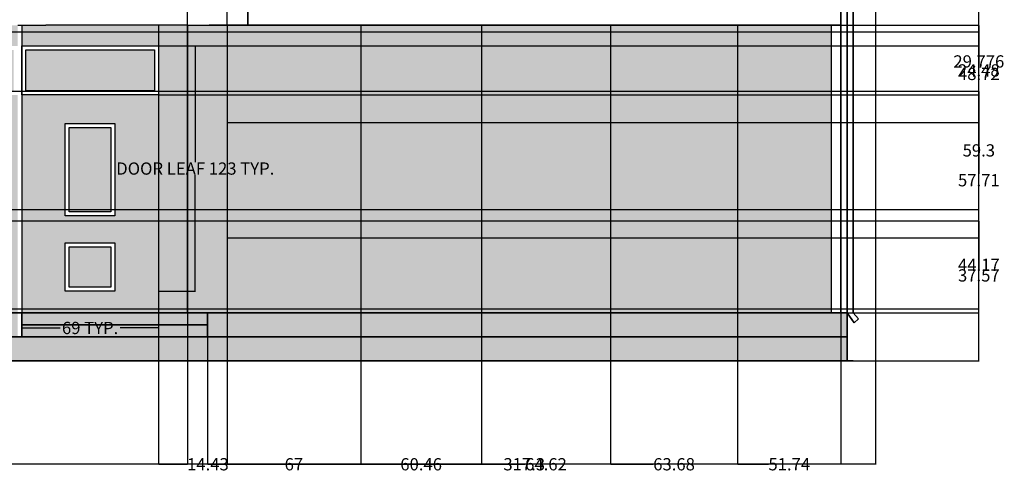
# Model space of a CAD drawing. Units: inches. Extents: x -655 to 499, y 20 to 616.
# Tile 6 of 7: x 5 to 499, y 20 to 246. Entities that reach past the tile are written whole.
import ezdxf

# ---------------------------------------------------------------- set-up
doc = ezdxf.new("R2010")
doc.units = ezdxf.units.IN
doc.header["$MEASUREMENT"] = 0
for name, color, linetype, lineweight in [('A-ANNO-DIMS', 2, 'Continuous', 18), ('A-DOOR', 4, 'Continuous', 25), ('A-ELEV', 7, 'Continuous', 35), ('A-ELEV-PATT', 9, 'Continuous', 13), ('A-GLAZ', 3, 'Continuous', 25), ('C-TOPO', 18, 'Continuous', 18)]:
    doc.layers.add(name, color=color, linetype=linetype, lineweight=lineweight)
doc.styles.get("Standard").update_dxf_attribs({"font": 'arial.ttf'})
doc.dimstyles.get("Standard").update_dxf_attribs({"dimtxt": 6.125, "dimasz": 0.18, "dimexe": 0.18, "dimexo": 0.0625, "dimgap": 0.09, "dimtad": 0, "dimtih": 1, "dimtoh": 1, "dimdec": 4, "dimzin": 0, "dimdsep": 46, "dimlunit": 4, "dimtxsty": 'Standard', "dimcen": 0.09, "dimadec": 0, "dimazin": 0, "dimtfac": 1, "dimtdec": 4, "dimtofl": 0, "dimtmove": 0, "dimatfit": 3, "dimfxl": 1, "dimtolj": 1, "dimtzin": 0, "dimarcsym": 0})

# ---------------------------------------------------------------- blocks, each defined once
blk = doc.blocks.new('DOOR-LEAF-PANEL')
for points in [[(0, 122.75), (68.54, 122.75), (68.54, 98.27), (0, 98.27)], [(2, 120.75), (66.54, 120.75), (66.54, 100.27), (2, 100.27)], [(21.82, 83.95), (46.58, 83.95), (46.58, 37.78), (21.82, 37.78)], [(23.82, 81.95), (44.58, 81.95), (44.58, 39.78), (23.82, 39.78)], [(21.82, 24.14), (46.58, 24.14), (46.58, 0), (21.82, 0)], [(23.82, 22.14), (44.58, 22.14), (44.58, 2), (23.82, 2)]]:
    blk.add_lwpolyline(points, close=True)
blk = doc.blocks.new('*D8')
at = {"layer": 'A-ANNO-DIMS', "color": 0, "lineweight": -2, "transparency": 16777216}
for p, q in [((75.03, 233.27), (93.56, 233.27)), ((93.38, 233.09), (93.38, 175.16)), ((93.38, 110.71), (93.38, 168.64)), ((75.03, 110.53), (93.56, 110.53))]:
    blk.add_line(p, q, dxfattribs=at)
at = {"layer": 'A-ANNO-DIMS', "color": 0, "transparency": 16777216}
for points in [[(93.35, 233.09), (93.41, 233.09), (93.38, 233.27)], [(93.35, 110.71), (93.41, 110.71), (93.38, 110.53)]]:
    blk.add_solid(points, dxfattribs=at)
at = {"layer": 'Defpoints', "color": 0, "transparency": 16777216}
for p in [(74.97, 233.27), (93.38, 233.27), (74.97, 110.53)]:
    blk.add_point(p, dxfattribs=at)
at = {"layer": 'A-ANNO-DIMS', "color": 0, "transparency": 16777216, "insert": (93.38, 171.9), "char_height": 6.125, "attachment_point": 5}
blk.add_mtext('\\A1;DOOR LEAF 123 TYP.', dxfattribs=at)
blk = doc.blocks.new('*D9')
at = {"layer": 'A-ANNO-DIMS', "color": 0, "lineweight": -2, "transparency": 16777216}
for p, q in [((6.43, 110.46), (6.43, 91.93)), ((74.97, 110.46), (74.97, 91.93)), ((6.61, 92.11), (25.68, 92.11)), ((74.79, 92.11), (55.71, 92.11))]:
    blk.add_line(p, q, dxfattribs=at)
at = {"layer": 'A-ANNO-DIMS', "color": 0, "transparency": 16777216}
for points in [[(6.61, 92.14), (6.61, 92.08), (6.43, 92.11)], [(74.79, 92.14), (74.79, 92.08), (74.97, 92.11)]]:
    blk.add_solid(points, dxfattribs=at)
at = {"layer": 'Defpoints', "color": 0, "transparency": 16777216}
for p in [(6.43, 110.53), (74.97, 110.53), (74.97, 92.11)]:
    blk.add_point(p, dxfattribs=at)
at = {"layer": 'A-ANNO-DIMS', "color": 0, "transparency": 16777216, "insert": (40.7, 92.11), "char_height": 6.125, "attachment_point": 5}
blk.add_mtext('\\A1;69 TYP.', dxfattribs=at)
blk = doc.blocks.new('*D10')
at = {"layer": 'A-ANNO-DIMS', "color": 0, "lineweight": -2, "transparency": 16777216}
for p, q in [((434.11, 393.11), (434.11, 23.7)), ((-590.16, 75.57), (-590.16, 23.7)), ((-589.98, 23.88), (-90.54, 23.88)), ((433.93, 23.88), (-65.51, 23.88))]:
    blk.add_line(p, q, dxfattribs=at)
at = {"layer": 'A-ANNO-DIMS', "color": 0, "transparency": 16777216}
for points in [[(-589.98, 23.91), (-589.98, 23.85), (-590.16, 23.88)], [(433.93, 23.91), (433.93, 23.85), (434.11, 23.88)]]:
    blk.add_solid(points, dxfattribs=at)
at = {"layer": 'Defpoints', "color": 0, "transparency": 16777216}
for p in [(434.11, 393.17), (-590.16, 75.63), (434.11, 23.88)]:
    blk.add_point(p, dxfattribs=at)
at = {"layer": 'A-ANNO-DIMS', "color": 0, "transparency": 16777216, "insert": (-78.02, 23.88), "char_height": 6.125, "attachment_point": 5}
blk.add_mtext('\\A1;1024.3', dxfattribs=at)
blk = doc.blocks.new('*D15')
at = {"layer": 'A-ANNO-DIMS', "color": 0, "lineweight": -2, "transparency": 16777216}
for p, q in [((-126.81, 99.57), (-126.81, 23.7)), ((99.5, 93.57), (99.5, 23.7)), ((-126.63, 23.88), (-24.13, 23.88)), ((99.32, 23.88), (-3.18, 23.88))]:
    blk.add_line(p, q, dxfattribs=at)
at = {"layer": 'A-ANNO-DIMS', "color": 0, "transparency": 16777216}
for points in [[(-126.63, 23.91), (-126.63, 23.85), (-126.81, 23.88)], [(99.32, 23.91), (99.32, 23.85), (99.5, 23.88)]]:
    blk.add_solid(points, dxfattribs=at)
at = {"layer": 'Defpoints', "color": 0, "transparency": 16777216}
for p in [(-126.81, 99.63), (99.5, 93.63), (99.5, 23.88)]:
    blk.add_point(p, dxfattribs=at)
at = {"layer": 'A-ANNO-DIMS', "color": 0, "transparency": 16777216, "insert": (-13.65, 23.88), "char_height": 6.125, "attachment_point": 5}
blk.add_mtext('\\A1;226.3', dxfattribs=at)
blk = doc.blocks.new('*D16')
at = {"layer": 'A-ANNO-DIMS', "color": 0, "lineweight": -2, "transparency": 16777216}
for p, q in [((416.78, 99.57), (416.78, 23.7)), ((99.5, 93.57), (99.5, 23.7)), ((99.68, 23.88), (247.71, 23.88)), ((416.6, 23.88), (268.56, 23.88))]:
    blk.add_line(p, q, dxfattribs=at)
at = {"layer": 'A-ANNO-DIMS', "color": 0, "transparency": 16777216}
for points in [[(99.68, 23.91), (99.68, 23.85), (99.5, 23.88)], [(416.6, 23.91), (416.6, 23.85), (416.78, 23.88)]]:
    blk.add_solid(points, dxfattribs=at)
at = {"layer": 'Defpoints', "color": 0, "transparency": 16777216}
for p in [(416.78, 99.63), (99.5, 93.63), (416.78, 23.88)]:
    blk.add_point(p, dxfattribs=at)
at = {"layer": 'A-ANNO-DIMS', "color": 0, "transparency": 16777216, "insert": (258.14, 23.88), "char_height": 6.125, "attachment_point": 5}
blk.add_mtext('\\A1;317.3', dxfattribs=at)
blk = doc.blocks.new('*D21')
at = {"layer": 'A-ANNO-DIMS', "color": 0, "lineweight": -2, "transparency": 16777216}
for p, q in [((179.11, 559.78), (486.04, 559.78)), ((485.86, 559.6), (485.86, 320.92)), ((485.86, 75.81), (485.86, 314.49)), ((-590.1, 75.63), (486.04, 75.63))]:
    blk.add_line(p, q, dxfattribs=at)
at = {"layer": 'A-ANNO-DIMS', "color": 0, "transparency": 16777216}
for points in [[(485.83, 559.6), (485.89, 559.6), (485.86, 559.78)], [(485.83, 75.81), (485.89, 75.81), (485.86, 75.63)]]:
    blk.add_solid(points, dxfattribs=at)
at = {"layer": 'Defpoints', "color": 0, "transparency": 16777216}
for p in [(179.05, 559.78), (485.86, 559.78), (-590.16, 75.63)]:
    blk.add_point(p, dxfattribs=at)
at = {"layer": 'A-ANNO-DIMS', "color": 0, "transparency": 16777216, "insert": (485.86, 317.7), "char_height": 6.125, "attachment_point": 5}
blk.add_mtext('\\A1;484.15', dxfattribs=at)
blk = doc.blocks.new('*D48')
at = {"layer": 'A-ANNO-DIMS', "color": 0, "lineweight": -2, "transparency": 16777216}
for p, q in [((-228.95, 145.8), (486.04, 145.8)), ((485.86, 145.62), (485.86, 126.88)), ((485.86, 101.81), (485.86, 120.55)), ((-228.95, 101.63), (486.04, 101.63))]:
    blk.add_line(p, q, dxfattribs=at)
at = {"layer": 'A-ANNO-DIMS', "color": 0, "transparency": 16777216}
for points in [[(485.83, 145.62), (485.89, 145.62), (485.86, 145.8)], [(485.83, 101.81), (485.89, 101.81), (485.86, 101.63)]]:
    blk.add_solid(points, dxfattribs=at)
at = {"layer": 'Defpoints', "color": 0, "transparency": 16777216}
for p in [(-229.01, 145.8), (485.86, 145.8), (-229.01, 101.63)]:
    blk.add_point(p, dxfattribs=at)
at = {"layer": 'A-ANNO-DIMS', "color": 0, "transparency": 16777216, "insert": (485.86, 123.72), "char_height": 6.125, "attachment_point": 5}
blk.add_mtext('\\A1;44.17', dxfattribs=at)
blk = doc.blocks.new('*D49')
at = {"layer": 'A-ANNO-DIMS', "color": 0, "lineweight": -2, "transparency": 16777216}
for p, q in [((-229.3, 210.64), (486.04, 210.64)), ((485.86, 210.46), (485.86, 184.21)), ((485.86, 151.52), (485.86, 177.77)), ((-229.3, 151.34), (486.04, 151.34))]:
    blk.add_line(p, q, dxfattribs=at)
at = {"layer": 'A-ANNO-DIMS', "color": 0, "transparency": 16777216}
for points in [[(485.83, 210.46), (485.89, 210.46), (485.86, 210.64)], [(485.83, 151.52), (485.89, 151.52), (485.86, 151.34)]]:
    blk.add_solid(points, dxfattribs=at)
at = {"layer": 'Defpoints', "color": 0, "transparency": 16777216}
for p in [(-229.36, 210.64), (485.86, 210.64), (-229.36, 151.34)]:
    blk.add_point(p, dxfattribs=at)
at = {"layer": 'A-ANNO-DIMS', "color": 0, "transparency": 16777216, "insert": (485.86, 180.99), "char_height": 6.125, "attachment_point": 5}
blk.add_mtext('\\A1;59.3', dxfattribs=at)
blk = doc.blocks.new('*D51')
at = {"layer": 'A-ANNO-DIMS', "color": 0, "lineweight": -2, "transparency": 16777216}
for p, q in [((-228.95, 240.42), (486.04, 240.42)), ((485.86, 240.24), (485.86, 228.75)), ((485.86, 210.82), (485.86, 222.31)), ((-228.88, 210.64), (486.04, 210.64))]:
    blk.add_line(p, q, dxfattribs=at)
at = {"layer": 'A-ANNO-DIMS', "color": 0, "transparency": 16777216}
for points in [[(485.83, 240.24), (485.89, 240.24), (485.86, 240.42)], [(485.83, 210.82), (485.89, 210.82), (485.86, 210.64)]]:
    blk.add_solid(points, dxfattribs=at)
at = {"layer": 'Defpoints', "color": 0, "transparency": 16777216}
for p in [(-229.01, 240.42), (485.86, 240.42), (-228.94, 210.64)]:
    blk.add_point(p, dxfattribs=at)
at = {"layer": 'A-ANNO-DIMS', "color": 0, "transparency": 16777216, "insert": (485.86, 225.53), "char_height": 6.125, "attachment_point": 5}
blk.add_mtext('\\A1;29.776', dxfattribs=at)
blk = doc.blocks.new('*D61')
at = {"layer": 'A-ANNO-DIMS', "color": 0, "lineweight": -2, "transparency": 16777216}
for p, q in [((-64.12, 233.34), (-64.12, 611.71)), ((89.4, 243.69), (89.4, 611.71)), ((-63.94, 611.53), (0.16, 611.53)), ((89.22, 611.53), (25.13, 611.53))]:
    blk.add_line(p, q, dxfattribs=at)
at = {"layer": 'A-ANNO-DIMS', "color": 0, "transparency": 16777216}
for points in [[(-63.94, 611.56), (-63.94, 611.5), (-64.12, 611.53)], [(89.22, 611.56), (89.22, 611.5), (89.4, 611.53)]]:
    blk.add_solid(points, dxfattribs=at)
at = {"layer": 'Defpoints', "color": 0, "transparency": 16777216}
for p in [(89.4, 611.53), (89.4, 243.63), (-64.12, 233.27)]:
    blk.add_point(p, dxfattribs=at)
at = {"layer": 'A-ANNO-DIMS', "color": 0, "transparency": 16777216, "insert": (12.64, 611.53), "char_height": 6.125, "attachment_point": 5}
blk.add_mtext('\\A1;153.52', dxfattribs=at)
blk = doc.blocks.new('*D62')
at = {"layer": 'A-ANNO-DIMS', "color": 0, "lineweight": -2, "transparency": 16777216}
for p, q in [((89.4, 243.69), (89.4, 611.71)), ((109.28, 243.69), (109.28, 611.71)), ((89.58, 611.53), (109.1, 611.53)), ((109.28, 611.53), (109.46, 611.53))]:
    blk.add_line(p, q, dxfattribs=at)
at = {"layer": 'A-ANNO-DIMS', "color": 0, "transparency": 16777216}
for points in [[(89.58, 611.56), (89.58, 611.5), (89.4, 611.53)], [(109.1, 611.56), (109.1, 611.5), (109.28, 611.53)]]:
    blk.add_solid(points, dxfattribs=at)
at = {"layer": 'Defpoints', "color": 0, "transparency": 16777216}
for p in [(109.28, 611.53), (89.4, 243.63), (109.28, 243.63)]:
    blk.add_point(p, dxfattribs=at)
at = {"layer": 'A-ANNO-DIMS', "color": 0, "transparency": 16777216, "insert": (121.99, 611.53), "char_height": 6.125, "attachment_point": 5}
blk.add_mtext('\\A1;19.875', dxfattribs=at)
blk = doc.blocks.new('*D63')
at = {"layer": 'A-ANNO-DIMS', "color": 0, "lineweight": -2, "transparency": 16777216}
for p, q in [((74.97, 99.57), (74.97, 23.7)), ((89.4, 99.57), (89.4, 23.7)), ((75.15, 23.88), (89.22, 23.88)), ((89.4, 23.88), (89.58, 23.88))]:
    blk.add_line(p, q, dxfattribs=at)
at = {"layer": 'A-ANNO-DIMS', "color": 0, "transparency": 16777216}
for points in [[(75.15, 23.91), (75.15, 23.85), (74.97, 23.88)], [(89.22, 23.91), (89.22, 23.85), (89.4, 23.88)]]:
    blk.add_solid(points, dxfattribs=at)
at = {"layer": 'Defpoints', "color": 0, "transparency": 16777216}
for p in [(74.97, 99.63), (89.4, 99.63), (89.4, 23.88)]:
    blk.add_point(p, dxfattribs=at)
at = {"layer": 'A-ANNO-DIMS', "color": 0, "transparency": 16777216, "insert": (99.72, 23.88), "char_height": 6.125, "attachment_point": 5}
blk.add_mtext('\\A1;14.43', dxfattribs=at)
blk = doc.blocks.new('*D64')
at = {"layer": 'A-ANNO-DIMS', "color": 0, "lineweight": -2, "transparency": 16777216}
for p, q in [((75.03, 233.27), (486.04, 233.27)), ((485.86, 233.09), (485.86, 224.25)), ((485.86, 208.97), (485.86, 217.82)), ((75.03, 208.79), (486.04, 208.79))]:
    blk.add_line(p, q, dxfattribs=at)
at = {"layer": 'A-ANNO-DIMS', "color": 0, "transparency": 16777216}
for points in [[(485.83, 233.09), (485.89, 233.09), (485.86, 233.27)], [(485.83, 208.97), (485.89, 208.97), (485.86, 208.79)]]:
    blk.add_solid(points, dxfattribs=at)
at = {"layer": 'Defpoints', "color": 0, "transparency": 16777216}
for p in [(74.97, 233.27), (485.86, 233.27), (74.97, 208.79)]:
    blk.add_point(p, dxfattribs=at)
at = {"layer": 'A-ANNO-DIMS', "color": 0, "transparency": 16777216, "insert": (485.86, 221.03), "char_height": 6.125, "attachment_point": 5}
blk.add_mtext('\\A1;24.48', dxfattribs=at)
blk = doc.blocks.new('*D72')
at = {"layer": 'A-ANNO-DIMS', "color": 0, "lineweight": -2, "transparency": 16777216}
for p, q in [((109.28, 243.57), (109.28, 23.7)), ((176.28, 243.57), (176.28, 23.7)), ((109.46, 23.88), (138.28, 23.88)), ((176.1, 23.88), (147.27, 23.88))]:
    blk.add_line(p, q, dxfattribs=at)
at = {"layer": 'A-ANNO-DIMS', "color": 0, "transparency": 16777216}
for points in [[(109.46, 23.91), (109.46, 23.85), (109.28, 23.88)], [(176.1, 23.91), (176.1, 23.85), (176.28, 23.88)]]:
    blk.add_solid(points, dxfattribs=at)
at = {"layer": 'Defpoints', "color": 0, "transparency": 16777216}
for p in [(109.28, 243.63), (176.28, 243.63), (176.28, 23.88)]:
    blk.add_point(p, dxfattribs=at)
at = {"layer": 'A-ANNO-DIMS', "color": 0, "transparency": 16777216, "insert": (142.78, 23.88), "char_height": 6.125, "attachment_point": 5}
blk.add_mtext('\\A1;67', dxfattribs=at)
blk = doc.blocks.new('*D73')
at = {"layer": 'A-ANNO-DIMS', "color": 0, "lineweight": -2, "transparency": 16777216}
for p, q in [((176.28, 243.57), (176.28, 23.7)), ((236.74, 243.57), (236.74, 23.7)), ((176.46, 23.88), (196.07, 23.88)), ((236.56, 23.88), (216.95, 23.88))]:
    blk.add_line(p, q, dxfattribs=at)
at = {"layer": 'A-ANNO-DIMS', "color": 0, "transparency": 16777216}
for points in [[(176.46, 23.91), (176.46, 23.85), (176.28, 23.88)], [(236.56, 23.91), (236.56, 23.85), (236.74, 23.88)]]:
    blk.add_solid(points, dxfattribs=at)
at = {"layer": 'Defpoints', "color": 0, "transparency": 16777216}
for p in [(176.28, 243.63), (236.74, 243.63), (236.74, 23.88)]:
    blk.add_point(p, dxfattribs=at)
at = {"layer": 'A-ANNO-DIMS', "color": 0, "transparency": 16777216, "insert": (206.51, 23.88), "char_height": 6.125, "attachment_point": 5}
blk.add_mtext('\\A1;60.46', dxfattribs=at)
blk = doc.blocks.new('*D74')
at = {"layer": 'A-ANNO-DIMS', "color": 0, "lineweight": -2, "transparency": 16777216}
for p, q in [((236.74, 243.57), (236.74, 23.7)), ((301.36, 243.57), (301.36, 23.7)), ((236.92, 23.88), (258.64, 23.88)), ((301.18, 23.88), (279.46, 23.88))]:
    blk.add_line(p, q, dxfattribs=at)
at = {"layer": 'A-ANNO-DIMS', "color": 0, "transparency": 16777216}
for points in [[(236.92, 23.91), (236.92, 23.85), (236.74, 23.88)], [(301.18, 23.91), (301.18, 23.85), (301.36, 23.88)]]:
    blk.add_solid(points, dxfattribs=at)
at = {"layer": 'Defpoints', "color": 0, "transparency": 16777216}
for p in [(236.74, 243.63), (301.36, 243.63), (301.36, 23.88)]:
    blk.add_point(p, dxfattribs=at)
at = {"layer": 'A-ANNO-DIMS', "color": 0, "transparency": 16777216, "insert": (269.05, 23.88), "char_height": 6.125, "attachment_point": 5}
blk.add_mtext('\\A1;64.62', dxfattribs=at)
blk = doc.blocks.new('*D75')
at = {"layer": 'A-ANNO-DIMS', "color": 0, "lineweight": -2, "transparency": 16777216}
for p, q in [((301.36, 243.57), (301.36, 23.7)), ((365.04, 243.57), (365.04, 23.7)), ((301.54, 23.88), (322.75, 23.88)), ((364.86, 23.88), (343.65, 23.88))]:
    blk.add_line(p, q, dxfattribs=at)
at = {"layer": 'A-ANNO-DIMS', "color": 0, "transparency": 16777216}
for points in [[(301.54, 23.91), (301.54, 23.85), (301.36, 23.88)], [(364.86, 23.91), (364.86, 23.85), (365.04, 23.88)]]:
    blk.add_solid(points, dxfattribs=at)
at = {"layer": 'Defpoints', "color": 0, "transparency": 16777216}
for p in [(301.36, 243.63), (365.04, 243.63), (365.04, 23.88)]:
    blk.add_point(p, dxfattribs=at)
at = {"layer": 'A-ANNO-DIMS', "color": 0, "transparency": 16777216, "insert": (333.2, 23.88), "char_height": 6.125, "attachment_point": 5}
blk.add_mtext('\\A1;63.68', dxfattribs=at)
blk = doc.blocks.new('*D76')
at = {"layer": 'A-ANNO-DIMS', "color": 0, "lineweight": -2, "transparency": 16777216}
for p, q in [((365.04, 243.57), (365.04, 23.7)), ((416.78, 243.57), (416.78, 23.7)), ((365.22, 23.88), (380.5, 23.88)), ((416.6, 23.88), (401.32, 23.88))]:
    blk.add_line(p, q, dxfattribs=at)
at = {"layer": 'A-ANNO-DIMS', "color": 0, "transparency": 16777216}
for points in [[(365.22, 23.91), (365.22, 23.85), (365.04, 23.88)], [(416.6, 23.91), (416.6, 23.85), (416.78, 23.88)]]:
    blk.add_solid(points, dxfattribs=at)
at = {"layer": 'Defpoints', "color": 0, "transparency": 16777216}
for p in [(365.04, 243.63), (416.78, 243.63), (416.78, 23.88)]:
    blk.add_point(p, dxfattribs=at)
at = {"layer": 'A-ANNO-DIMS', "color": 0, "transparency": 16777216, "insert": (390.91, 23.88), "char_height": 6.125, "attachment_point": 5}
blk.add_mtext('\\A1;51.74', dxfattribs=at)
blk = doc.blocks.new('*D77')
at = {"layer": 'A-ANNO-DIMS', "color": 0, "lineweight": -2, "transparency": 16777216}
for p, q in [((412.05, 137.2), (486.04, 137.2)), ((485.86, 137.02), (485.86, 121.63)), ((485.86, 99.81), (485.86, 115.2)), ((416.84, 99.63), (486.04, 99.63))]:
    blk.add_line(p, q, dxfattribs=at)
at = {"layer": 'A-ANNO-DIMS', "color": 0, "transparency": 16777216}
for points in [[(485.83, 137.02), (485.89, 137.02), (485.86, 137.2)], [(485.83, 99.81), (485.89, 99.81), (485.86, 99.63)]]:
    blk.add_solid(points, dxfattribs=at)
at = {"layer": 'Defpoints', "color": 0, "transparency": 16777216}
for p in [(411.99, 137.2), (485.86, 137.2), (416.78, 99.63)]:
    blk.add_point(p, dxfattribs=at)
at = {"layer": 'A-ANNO-DIMS', "color": 0, "transparency": 16777216, "insert": (485.86, 118.41), "char_height": 6.125, "attachment_point": 5}
blk.add_mtext('\\A1;37.57', dxfattribs=at)
blk = doc.blocks.new('*D78')
at = {"layer": 'A-ANNO-DIMS', "color": 0, "lineweight": -2, "transparency": 16777216}
for p, q in [((412.05, 194.91), (486.04, 194.91)), ((485.86, 194.73), (485.86, 169.27)), ((485.86, 137.38), (485.86, 162.84)), ((412.05, 137.2), (486.04, 137.2))]:
    blk.add_line(p, q, dxfattribs=at)
at = {"layer": 'A-ANNO-DIMS', "color": 0, "transparency": 16777216}
for points in [[(485.83, 194.73), (485.89, 194.73), (485.86, 194.91)], [(485.83, 137.38), (485.89, 137.38), (485.86, 137.2)]]:
    blk.add_solid(points, dxfattribs=at)
at = {"layer": 'Defpoints', "color": 0, "transparency": 16777216}
for p in [(411.99, 194.91), (485.86, 194.91), (411.99, 137.2)]:
    blk.add_point(p, dxfattribs=at)
at = {"layer": 'A-ANNO-DIMS', "color": 0, "transparency": 16777216, "insert": (485.86, 166.06), "char_height": 6.125, "attachment_point": 5}
blk.add_mtext('\\A1;57.71', dxfattribs=at)
blk = doc.blocks.new('*D79')
at = {"layer": 'A-ANNO-DIMS', "color": 0, "lineweight": -2, "transparency": 16777216}
for p, q in [((416.84, 243.63), (486.04, 243.63)), ((485.86, 243.45), (485.86, 222.49)), ((485.86, 195.09), (485.86, 216.05)), ((412.05, 194.91), (486.04, 194.91))]:
    blk.add_line(p, q, dxfattribs=at)
at = {"layer": 'A-ANNO-DIMS', "color": 0, "transparency": 16777216}
for points in [[(485.83, 243.45), (485.89, 243.45), (485.86, 243.63)], [(485.83, 195.09), (485.89, 195.09), (485.86, 194.91)]]:
    blk.add_solid(points, dxfattribs=at)
at = {"layer": 'Defpoints', "color": 0, "transparency": 16777216}
for p in [(416.78, 243.63), (485.86, 243.63), (411.99, 194.91)]:
    blk.add_point(p, dxfattribs=at)
at = {"layer": 'A-ANNO-DIMS', "color": 0, "transparency": 16777216, "insert": (485.86, 219.27), "char_height": 6.125, "attachment_point": 5}
blk.add_mtext('\\A1;48.72', dxfattribs=at)
blk = doc.blocks.new('*D80')
at = {"layer": 'A-ANNO-DIMS', "color": 0, "lineweight": -2, "transparency": 16777216}
for p, q in [((270.7, 282.96), (486.04, 282.96)), ((485.86, 282.78), (485.86, 266.51)), ((485.86, 243.81), (485.86, 260.07)), ((416.84, 243.63), (486.04, 243.63))]:
    blk.add_line(p, q, dxfattribs=at)
at = {"layer": 'A-ANNO-DIMS', "color": 0, "transparency": 16777216}
for points in [[(485.83, 282.78), (485.89, 282.78), (485.86, 282.96)], [(485.83, 243.81), (485.89, 243.81), (485.86, 243.63)]]:
    blk.add_solid(points, dxfattribs=at)
at = {"layer": 'Defpoints', "color": 0, "transparency": 16777216}
for p in [(270.64, 282.96), (485.86, 282.96), (416.78, 243.63)]:
    blk.add_point(p, dxfattribs=at)
at = {"layer": 'A-ANNO-DIMS', "color": 0, "transparency": 16777216, "insert": (485.86, 263.29), "char_height": 6.125, "attachment_point": 5}
blk.add_mtext('\\A1;39.33', dxfattribs=at)

msp = doc.modelspace()

# ---------------------------------------------------------------- hatches: boundary and pattern name
at = {"layer": 'A-ELEV-PATT'}
h = msp.add_hatch(color=256, dxfattribs=at)
h.dxf.hatch_style = 1
h.paths.add_polyline_path([(-140.0489, 272.2618), (-399.3758, 272.2618), (-399.3758, 249.8418), (-399.3758, 248.5179), (-366.9446, 248.7444), (-209.8047, 249.8418), (-183.5755, 249.8418), (-140.0489, 249.8418)])
h.paths.add_polyline_path([(-211.7589, 317.0515), (-216.5713, 317.0515), (-216.5713, 272.2618), (-211.7589, 272.2618)])
h.paths.add_polyline_path([(-145.96, 317.0515), (-150.7725, 317.0515), (-150.7725, 272.2618), (-145.96, 272.2618)])
h.paths.add_polyline_path([(-140.5198, 321.4867), (-402.0739, 321.4867), (-402.0739, 317.0515), (-390.1757, 317.0515), (-385.3633, 317.0515), (-150.7725, 317.0515), (-145.96, 317.0515), (-140.5198, 317.0515)])
h.paths.add_polyline_path([(-269.7123, 317.0515), (-274.5248, 317.0515), (-274.5248, 272.2618), (-269.7123, 272.2618)])
h.paths.add_polyline_path([(-329.7837, 317.0515), (-334.5961, 317.0515), (-334.5961, 280.9678), (-329.7837, 280.9678)])
h.paths.add_polyline_path([(-329.7837, 280.9678), (-334.5961, 280.9678), (-334.5961, 272.2618), (-329.7837, 272.2618)])
h.paths.add_polyline_path([(-385.3633, 317.0515), (-390.1757, 317.0515), (-390.1757, 272.2618), (-385.3633, 272.2618)])
h.paths.add_polyline_path([(-229.0087, 240.4184), (-354.3532, 240.4184), (-354.2854, 210.6425), (-315.9956, 210.6425), (-315.9956, 210.9348), (-277.6793, 210.7995), (-277.6793, 210.6425), (-273.1052, 210.6425), (-273.1052, 210.7995), (-229.3637, 210.6425), (-229.0087, 210.6425)])
h.paths.add_polyline_path([(-229.0087, 145.8007), (-354.3532, 145.8007), (-354.3532, 101.6296), (-229.0087, 101.6296)])
h.paths.add_polyline_path([(-229.0087, 210.6425), (-229.3637, 210.6425), (-229.3637, 151.3385), (-273.1052, 151.4955), (-273.1052, 210.6425), (-277.6793, 210.6425), (-277.6793, 151.4955), (-315.9956, 151.6308), (-315.9956, 210.6425), (-318.9742, 210.6425), (-318.9742, 151.3385), (-354.3532, 151.3385), (-354.3532, 145.8007), (-229.0087, 145.8007)])
h.paths.add_polyline_path([(-229.0087, 247.8418), (-354.3532, 247.8418), (-354.3532, 240.4184), (-229.0087, 240.4184)])
h.paths.add_polyline_path([(4.4271, 93.6296), (-100.4134, 93.6296), (-124.8077, 93.6296), (-126.8077, 93.6296), (-126.8077, 87.6296), (4.4271, 87.6296)])
h.paths.add_polyline_path([(4.4271, 99.6296), (-100.4134, 99.6296), (-100.4134, 93.6296), (4.4271, 93.6296)])
h.paths.add_polyline_path([(99.4982, 99.6296), (6.4271, 99.6296), (6.4271, 93.6296), (99.4982, 93.6296)])
h.paths.add_polyline_path([(99.4982, 93.6296), (6.4271, 93.6296), (6.4271, 87.6296), (99.4982, 87.6296)])
h.paths.add_polyline_path([(304.2843, 311.436), (230.0144, 311.076), (230.0144, 282.9577), (270.6361, 282.9577), (304.4665, 273.8535)])
h.paths.add_polyline_path([(304.1054, 348.3371), (304.1054, 356.2861), (230.0144, 356.2861), (230.0144, 348.3443), (230.0144, 311.076), (304.2843, 311.436)])
h.paths.add_polyline_path([(255.5586, 316.5111), (255.5586, 350.0185), (275.6848, 350.0185), (275.6848, 316.5111)], flags=16)
h.paths.add_polyline_path([(278.0676, 316.5111), (278.0676, 350.0185), (301.4074, 350.0185), (301.4074, 316.5111)], flags=16)
h.paths.add_polyline_path([(253.2029, 316.5111), (233.8107, 316.5111), (233.8107, 350.0185), (253.2029, 350.0185)], flags=16)
h.paths.add_polyline_path([(179.0482, 559.7795), (153.2347, 535.8185), (165.0976, 535.8185), (192.9989, 535.8185), (201.2897, 535.8185)])
h.paths.add_polyline_path([(347.8163, 516.7932), (322.0028, 492.8322), (333.8657, 492.8322), (361.7669, 492.8322), (370.0577, 492.8322)])
h = msp.add_hatch(color=256, dxfattribs=at)
h.dxf.hatch_style = 1
h.paths.add_polyline_path([(-329.7837, 350.1333), (-347.0336, 350.1333), (-347.0336, 321.4867), (-329.7837, 321.4867)])
h.paths.add_polyline_path([(-294.1413, 350.1333), (-311.3912, 350.1333), (-311.3912, 321.4867), (-294.1413, 321.4867)])
h.paths.add_polyline_path([(-294.1413, 317.0515), (-311.3912, 317.0515), (-311.3912, 280.9678), (-294.1413, 280.9678)])
h.paths.add_polyline_path([(-334.5961, 317.0515), (-347.0336, 317.0515), (-347.0336, 280.9678), (-334.5961, 280.9678)])
h.paths.add_polyline_path([(-244.6859, 336.719), (-258.4486, 336.719), (-258.4486, 347.0139), (-244.6859, 347.0139), (-244.6859, 350.1333), (-261.9358, 350.1333), (-261.9358, 321.4867), (-244.6859, 321.4867)])
h.paths.add_polyline_path([(-244.6859, 317.0515), (-261.9358, 317.0515), (-261.9358, 280.9678), (-244.6859, 280.9678)])
h.paths.add_polyline_path([(-244.6859, 347.0139), (-258.4486, 347.0139), (-258.4486, 336.719), (-244.6859, 336.719)], flags=17)
h.paths.add_polyline_path([(-318.9742, 210.6425), (-354.3532, 210.6425), (-354.3532, 151.3385), (-318.9742, 151.3385)])
h.paths.add_polyline_path([(-277.6793, 210.6425), (-315.9956, 210.6425), (-315.9956, 151.6308), (-277.6793, 151.4955)])
h.paths.add_polyline_path([(-229.3637, 210.6425), (-273.1052, 210.6425), (-273.1052, 151.4955), (-229.3637, 151.3385)])
h.paths.add_polyline_path([(-19.537, 192.4712), (-40.2951, 192.4712), (-40.2951, 150.3082), (-19.537, 150.3082)])
h.paths.add_polyline_path([(2.4271, 231.274), (-62.1158, 231.274), (-62.1158, 210.7923), (2.4271, 210.7923)])
h.paths.add_polyline_path([(72.97, 231.274), (8.4271, 231.274), (8.4271, 210.7923), (72.97, 210.7923)])
h.paths.add_polyline_path([(51.0059, 192.4712), (30.2478, 192.4712), (30.2478, 150.3082), (51.0059, 150.3082)])
h.paths.add_polyline_path([(51.0059, 132.6671), (30.2478, 132.6671), (30.2478, 112.5254), (51.0059, 112.5254)])
h.paths.add_polyline_path([(-19.537, 132.6671), (-40.2951, 132.6671), (-40.2951, 112.5254), (-19.537, 112.5254)])
h.paths.add_polyline_path([(275.6848, 350.0185), (255.5586, 350.0185), (255.5586, 316.5111), (275.6848, 316.5111)])
h.paths.add_polyline_path([(301.4074, 350.0185), (278.0676, 350.0185), (278.0676, 316.5111), (301.4074, 316.5111)])
h.paths.add_polyline_path([(253.2029, 350.0185), (233.8107, 350.0185), (233.8107, 316.5111), (253.2029, 316.5111)])
h = msp.add_hatch(color=256, dxfattribs=at)
h.dxf.hatch_style = 1
h.paths.add_polyline_path([(-150.7725, 317.0515), (-211.7589, 317.0515), (-211.7589, 272.2618), (-150.7725, 272.2618)])
h.paths.add_polyline_path([(-229.0087, 317.0515), (-244.6859, 317.0515), (-244.6859, 280.9678), (-261.9358, 280.9678), (-261.9358, 317.0515), (-269.7123, 317.0515), (-269.7123, 272.2618), (-229.0087, 272.2618)])
h.paths.add_polyline_path([(-216.5713, 317.0515), (-227.0087, 317.0515), (-227.0087, 272.2618), (-216.5713, 272.2618)])
h.paths.add_polyline_path([(-274.5248, 317.0515), (-294.1413, 317.0515), (-294.1413, 280.9678), (-311.3912, 280.9678), (-311.3912, 317.0515), (-329.7837, 317.0515), (-329.7837, 280.9678), (-329.7837, 272.2618), (-274.5248, 272.2618)])
h.paths.add_polyline_path([(-347.0336, 317.0515), (-355.429, 317.0515), (-355.429, 272.2618), (-334.5961, 272.2618), (-334.5961, 280.9678), (-347.0336, 280.9678)])
h.paths.add_polyline_path([(-357.429, 317.0515), (-385.3633, 317.0515), (-385.3633, 272.2618), (-357.429, 272.2618)])
h.paths.add_polyline_path([(176.2798, 243.6296), (109.2763, 243.6296), (109.2763, 194.9112), (176.2798, 194.9112)])
h.paths.add_polyline_path([(176.2798, 194.9112), (109.2763, 194.9112), (109.2763, 137.2003), (176.2798, 137.2003)])
h.paths.add_polyline_path([(236.7365, 243.6296), (176.2798, 243.6296), (176.2798, 194.9112), (236.7365, 194.9112)])
h.paths.add_polyline_path([(236.7365, 194.9112), (176.2798, 194.9112), (176.2798, 137.2003), (236.7365, 137.2003)])
h.paths.add_polyline_path([(236.7365, 137.2003), (176.2798, 137.2003), (176.2798, 99.6296), (236.7365, 99.6296)])
h.paths.add_polyline_path([(176.2798, 137.2003), (109.2763, 137.2003), (109.2763, 99.6296), (176.2798, 99.6296)])
h.paths.add_polyline_path([(301.3566, 137.2003), (236.7365, 137.2003), (236.7365, 99.6296), (301.3566, 99.6296)])
h.paths.add_polyline_path([(301.3566, 194.9112), (236.7365, 194.9112), (236.7365, 137.2003), (301.3566, 137.2003)])
h.paths.add_polyline_path([(301.3566, 243.6296), (236.7365, 243.6296), (236.7365, 194.9112), (301.3566, 194.9112)])
h.paths.add_polyline_path([(365.0401, 243.6296), (301.3566, 243.6296), (301.3566, 194.9112), (365.0401, 194.9112)])
h.paths.add_polyline_path([(365.0401, 194.9112), (301.3566, 194.9112), (301.3566, 137.2003), (365.0401, 137.2003)])
h.paths.add_polyline_path([(411.9901, 243.6296), (365.0401, 243.6296), (365.0401, 194.9112), (411.9901, 194.9112)])
h.paths.add_polyline_path([(411.9901, 194.9112), (365.0401, 194.9112), (365.0401, 99.6296), (411.9901, 99.6296)])
h.paths.add_polyline_path([(365.0401, 137.2003), (301.3566, 137.2003), (301.3566, 99.6296), (365.0401, 99.6296)])
h = msp.add_hatch(color=256, dxfattribs=at)
h.dxf.hatch_style = 1
h.paths.add_polyline_path([(-126.8077, 93.6296), (-126.8077, 99.6296), (-145.6102, 99.6296), (-209.8047, 99.6296), (-366.9446, 98.5321), (-366.9446, 99.6296), (-506.835, 99.6296), (-573.6788, 99.6296), (-573.6788, 87.6296), (-506.835, 87.6296), (-161.7817, 87.6296), (-126.8077, 87.6296)])
h.paths.add_polyline_path([(419.8436, 99.6296), (99.4982, 99.6296), (99.4982, 87.6296), (419.8436, 87.6296)])
h.paths.add_polyline_path([(-100.4134, 99.6296), (-124.8077, 99.6296), (-124.8077, 93.6296), (-100.4134, 93.6296)])
h.paths.add_polyline_path([(-124.8077, 243.6296), (-126.8077, 243.6296), (-126.8077, 99.6296), (-124.8077, 99.6296)])
h.paths.add_polyline_path([(-124.8077, 99.6296), (-126.8077, 99.6296), (-126.8077, 93.6296), (-124.8077, 93.6296)])
h = msp.add_hatch(color=256, dxfattribs=at)
h.dxf.hatch_style = 1
h.paths.add_polyline_path([(-78.9669, 243.6296), (-124.8077, 243.6296), (-124.8077, 99.6296), (-78.9669, 99.6296)])
h.paths.add_polyline_path([(109.2763, 243.6296), (100.3937, 243.6296), (89.4008, 243.6296), (89.4008, 99.6296), (99.4982, 99.6296), (109.2763, 99.6296)])
h = msp.add_hatch(color=256, dxfattribs=at)
h.dxf.hatch_style = 1
h.paths.add_polyline_path([(-64.1158, 243.6296), (-78.9669, 243.6296), (-78.9669, 99.6296), (-64.1158, 99.6296)])
h.paths.add_polyline_path([(74.97, 243.6296), (18.4987, 243.6296), (6.4271, 243.6296), (6.4271, 233.274), (74.97, 233.274)])
h.paths.add_polyline_path([(4.4271, 243.6296), (4.3518, 243.6296), (4.0451, 243.6296), (-52.0442, 243.6296), (-64.1158, 243.6296), (-64.1158, 233.274), (4.4271, 233.274)])
h.paths.add_polyline_path([(89.4008, 243.6296), (74.97, 243.6296), (74.97, 233.274), (74.97, 99.6296), (89.4008, 99.6296)])
h.paths.add_polyline_path([(74.97, 208.7923), (6.4271, 208.7923), (6.4271, 99.6296), (74.97, 99.6296)])
h.paths.add_polyline_path([(53.0059, 148.3082), (28.2478, 148.3082), (28.2478, 194.4712), (53.0059, 194.4712)], flags=16)
h.paths.add_polyline_path([(51.0059, 150.3082), (30.2478, 150.3082), (30.2478, 192.4712), (51.0059, 192.4712)], flags=0)
h.paths.add_polyline_path([(53.0059, 134.6671), (53.0059, 110.5254), (28.2478, 110.5254), (28.2478, 134.6671)], flags=16)
h.paths.add_polyline_path([(51.0059, 132.6671), (51.0059, 112.5254), (30.2478, 112.5254), (30.2478, 132.6671)], flags=0)
h.paths.add_polyline_path([(4.4271, 208.7923), (-64.1158, 208.7923), (-64.1158, 99.6296), (4.4271, 99.6296)])
h.paths.add_polyline_path([(-17.537, 148.3082), (-42.2951, 148.3082), (-42.2951, 194.4712), (-17.537, 194.4712)], flags=16)
h.paths.add_polyline_path([(-19.537, 150.3082), (-40.2951, 150.3082), (-40.2951, 192.4712), (-19.537, 192.4712)], flags=0)
h.paths.add_polyline_path([(-17.537, 134.6671), (-17.537, 110.5254), (-42.2951, 110.5254), (-42.2951, 134.6671)], flags=16)
h.paths.add_polyline_path([(-19.537, 132.6671), (-19.537, 112.5254), (-40.2951, 112.5254), (-40.2951, 132.6671)], flags=0)
at = {"layer": 'C-TOPO'}
h = msp.add_hatch(dxfattribs=at)
h.set_pattern_fill('GRAVEL', color=256, scale=2.2)
h.set_pattern_definition([(228.012788, (1.584, 2.2), (-17.6, -19.8), [0.295979, -29.301994]), (184.96974, (1.386, 1.98), (26.4, 2.2), [0.5079096, -50.2830345]), (132.510447, (0.88, 1.936), (22, -24.2), [0.3581336, -35.455272]), (267.27369, (0.022, 1.386), (2.2, 44), [0.4625236, -45.789828]), (292.833654, (0, 0.924), (-11, 26.4), [0.453541, -44.900621]), (357.27369, (0.176, 0.506), (-44, 2.2), [0.4625236, -45.789828]), (37.69424, (0.638, 0.484), (-28.6, -22), [0.611664, -60.554667]), (72.255328, (1.122, 0.858), (15.4, 48.4), [0.5774736, -57.169907]), (121.429566, (1.298, 1.408), (-17.6, 28.6), [0.46409, -45.944961]), (175.23636, (1.056, 1.804), (24.2, -2.2), [0.5298304, -25.961678]), (222.397438, (0.528, 1.848), (-26.4, -24.2), [0.6851856, -67.833425]), (138.814075, (2.2, 1.364), (-15.4, 13.2), [0.233862, -23.1524586]), (171.469234, (2.024, 1.518), (28.6, -4.4), [0.4449214, -44.047325]), (225, (1.584, 1.584), (-2e-16, -2.2), [0.311126, -2.800144]), (203.19859, (1.43, 1.848), (11, 4.4), [0.1675476, -16.587153]), (291.80141, (1.276, 1.782), (-2.2, 6.6), [0.2369466, -11.610416]), (30.96376, (1.364, 1.562), (6.6, 4.4), [0.384844, -12.44325]), (161.56505, (1.694, 1.76), (4.4, -2.2), [0.27828, -6.678731]), (16.38954, (0, 1.782), (22, 6.6), [0.38984, -38.594259]), (70.346176, (0.374, 1.892), (-8.8, -24.2), [0.327054, -32.378297]), (293.19859, (1.694, 2.2), (-4.4, 11), [0.335093, -16.419608]), (343.61046, (1.826, 1.892), (-22, 6.6), [0.38984, -38.594259]), (339.443955, (0, 0.418), (-11, 4.4), [0.375936, -18.420872]), (294.77514, (0.352, 0.286), (-11, 24.2), [0.3149916, -31.184215]), (66.80141, (1.716, 0), (4.4, 11), [0.335093, -16.419608]), (17.354025, (1.848, 0.308), (-28.6, -8.8), [0.368788, -36.509932]), (69.443955, (0.638, 0), (-4.4, -11), [0.187968, -18.60884]), (101.30993, (1.584, 0), (-2.2, 8.8), [0.112178, -11.105665]), (165.96376, (1.562, 0.11), (6.6, -2.2), [0.453541, -8.617291]), (186.009006, (1.122, 0.22), (22, 2.2), [0.42031, -41.610631]), (303.69007, (1.364, 1.364), (-2.2, 4.4), [0.3172884, -7.6149244]), (353.157227, (1.54, 1.1), (37.4, -4.4), [0.553947, -54.840638]), (60.945396, (2.09, 1.034), (-8.8, -15.4), [0.226503, -22.423883]), (90, (2.2, 1.232), (-2.2, 2.2), [0.132, -2.068]), (120.256437, (1.078, 0.286), (8.8, -15.4), [0.305633, -30.257744]), (48.012788, (0.924, 0.55), (17.6, 19.8), [0.5919584, -29.0060145]), (0, (1.32, 0.99), (2.2, 2.2), [0.572, -1.628]), (325.304846, (1.892, 0.99), (22, -15.4), [0.347851, -34.4372035]), (254.054604, (2.178, 0.792), (-2.2, -8.8), [0.3203244, -15.695917]), (207.645975, (2.09, 0.484), (-41.8, -22), [0.521543, -51.632843]), (175.426079, (1.628, 0.242), (-28.6, 2.2), [0.551758, -54.6239615])])
h.paths.add_polyline_path([(419.8436, 87.6296), (99.4982, 87.6296), (-161.7817, 87.6296), (-506.835, 87.6296), (-573.6788, 87.6296), (-590.1625, 87.6296), (-590.1625, 75.6296), (-496.5301, 75.6296), (-76.7836, 75.6296), (99.4982, 75.6296), (419.8436, 75.6296)])

# ---------------------------------------------------------------- linework, layer by layer
at = {"layer": 'A-DOOR'}
for p, q in [((4.4271, 243.6296), (6.4271, 243.6296)), ((6.4271, 243.6296), (6.4271, 99.6296)), ((6.4271, 243.6296), (18.4987, 243.6296)), ((89.4008, 243.6296), (18.4987, 243.6296)), ((74.97, 243.6296), (74.97, 99.6296)), ((89.4008, 243.6296), (100.3937, 243.6296))]:
    msp.add_line(p, q, dxfattribs=at)
at = {"layer": 'A-ELEV'}
for p, q in [((416.7758, 243.6296), (416.7463, 390.1653)), ((119.638, 243.6296), (119.638, 387.6296)), ((419.8436, 99.6296), (419.8436, 373.8555)), ((422.8436, 99.6296), (422.8436, 373.8964)), ((89.4008, 243.6296), (89.4008, 99.6296)), ((416.7758, 243.6296), (100.3937, 243.6296)), ((416.7758, 243.6296), (416.7758, 99.6296)), ((99.4982, 99.6296), (-145.6102, 99.6296)), ((6.4271, 99.6296), (6.4271, 87.6296)), ((99.4982, 99.6296), (419.8436, 99.6296)), ((99.4982, 99.6296), (99.4982, 87.6296)), ((419.8436, 87.6296), (419.8436, 99.6296)), ((423.4661, 94.7015), (419.8436, 99.6296)), ((422.8436, 99.6296), (425.6043, 96.7554)), ((425.6043, 96.7554), (423.4661, 94.7015)), ((6.4271, 93.6296), (99.4982, 93.6296)), ((99.4982, 87.6296), (-161.7817, 87.6296)), ((99.4982, 87.6296), (419.8436, 87.6296)), ((419.8436, 75.6296), (419.8436, 87.6296)), ((99.4982, 75.6296), (-76.7836, 75.6296)), ((99.4982, 75.6296), (419.8436, 75.6296)), ((422.8436, 75.6296), (419.8436, 75.6296))]:
    msp.add_line(p, q, dxfattribs=at)
at = {"layer": 'A-GLAZ'}
for p, q in [((176.2798, 243.6296), (176.2798, 99.6296)), ((236.7365, 243.6296), (236.7365, 99.6296)), ((301.3566, 243.6296), (301.3566, 99.6296)), ((365.0401, 243.6296), (365.0401, 99.6296)), ((109.2763, 194.9112), (411.9901, 194.9112)), ((109.2763, 137.2003), (411.9901, 137.2003))]:
    msp.add_line(p, q, dxfattribs=at)
msp.add_lwpolyline([(411.9901, 243.6296), (109.2763, 243.6296), (109.2763, 99.6296), (411.9901, 99.6296)], close=True, dxfattribs=at)

# ---------------------------------------------------------------- block references
at = {"layer": 'A-DOOR'}
msp.add_blockref('DOOR-LEAF-PANEL', (6.427, 110.525), dxfattribs=at)

# ---------------------------------------------------------------- dimensions: what is measured, and where the dimension line sits
at = {"layer": 'A-ANNO-DIMS'}
for base, p1, p2, override, picture, middle in [((89.4008, 611.5295), (-64.1158, 233.274), (89.4008, 243.6296), {"dimdec": 2, "dimlfac": 1, "dimrnd": 0, "dimzin": 0, "dimdsep": 46, "dimlunit": 2}, '*D61', (12.6425, 611.5295)), ((109.27634, 611.52951), (89.40085, 243.6296), (109.27634, 243.6296), {"dimdec": 3, "dimlfac": 1, "dimrnd": 0, "dimzin": 0, "dimdsep": 46, "dimlunit": 2}, '*D62', (121.99479, 611.52951)), ((434.1137, 23.8796), (-590.1625, 75.6296), (434.1137, 393.1688), {"dimdec": 1, "dimlfac": 1, "dimrnd": 0, "dimzin": 0, "dimdsep": 46, "dimlunit": 2}, '*D10', (-78.0244, 23.8796)), ((176.2798, 23.8796), (109.2763, 243.6296), (176.2798, 243.6296), {"dimdec": 0, "dimlfac": 1, "dimrnd": 0, "dimzin": 0, "dimdsep": 46, "dimlunit": 2}, '*D72', (142.7781, 23.8796)), ((236.7365, 23.8796), (176.2798, 243.6296), (236.7365, 243.6296), {"dimdec": 2, "dimlfac": 1, "dimrnd": 0, "dimzin": 0, "dimdsep": 46, "dimlunit": 2}, '*D73', (206.5082, 23.8796)), ((301.3566, 23.8796), (236.7365, 243.6296), (301.3566, 243.6296), {"dimdec": 2, "dimlfac": 1, "dimrnd": 0, "dimzin": 0, "dimdsep": 46, "dimlunit": 2}, '*D74', (269.0466, 23.8796)), ((365.0401, 23.8796), (301.3566, 243.6296), (365.0401, 243.6296), {"dimdec": 2, "dimlfac": 1, "dimrnd": 0, "dimzin": 0, "dimdsep": 46, "dimlunit": 2}, '*D75', (333.1984, 23.8796)), ((416.7758, 23.8796), (365.0401, 243.6296), (416.7758, 243.6296), {"dimdec": 2, "dimlfac": 1, "dimrnd": 0, "dimzin": 0, "dimdsep": 46, "dimlunit": 2}, '*D76', (390.908, 23.8796)), ((99.4982, 23.8796), (-126.8077, 99.6296), (99.4982, 93.6296), {"dimdec": 1, "dimlfac": 1, "dimrnd": 0, "dimzin": 0, "dimdsep": 46, "dimlunit": 2}, '*D15', (-13.6547, 23.8796)), ((89.4008, 23.8796), (74.97, 99.6296), (89.4008, 99.6296), {"dimdec": 2, "dimlfac": 1, "dimrnd": 0, "dimzin": 0, "dimdsep": 46, "dimlunit": 2}, '*D63', (99.7169, 23.8796)), ((416.7758, 23.8796), (99.4982, 93.6296), (416.7758, 99.6296), {"dimdec": 1, "dimlfac": 1, "dimrnd": 0, "dimzin": 0, "dimdsep": 46, "dimlunit": 2}, '*D16', (258.137, 23.8796))]:
    dim = msp.add_linear_dim(base=base, p1=p1, p2=p2, dimstyle='Standard', override=override, dxfattribs=at)
    dim.commit()
    dim.dimension.update_dxf_attribs({"geometry": picture, "text_midpoint": middle})
for base, p1, p2, override, picture, middle in [((485.8637, 559.7795), (-590.1625, 75.6296), (179.0482, 559.7795), {"dimdec": 2, "dimlfac": 1, "dimrnd": 0, "dimzin": 0, "dimdsep": 46, "dimlunit": 2}, '*D21', (485.8637, 317.7046)), ((485.8637, 282.9577), (416.7758, 243.6296), (270.6361, 282.9577), {"dimdec": 2, "dimlfac": 1, "dimrnd": 0, "dimzin": 0, "dimdsep": 46, "dimlunit": 2}, '*D80', (485.8637, 263.2937)), ((485.8637, 243.6296), (411.9901, 194.9112), (416.7758, 243.6296), {"dimdec": 2, "dimlfac": 1, "dimrnd": 0, "dimzin": 0, "dimdsep": 46, "dimlunit": 2}, '*D79', (485.8637, 219.2704)), ((485.8637, 240.4184), (-228.941, 210.6425), (-229.0087, 240.4184), {"dimdec": 3, "dimlfac": 1, "dimrnd": 0, "dimzin": 0, "dimdsep": 46, "dimlunit": 2}, '*D51', (485.8637, 225.5305)), ((485.8637, 233.274), (74.97, 208.7923), (74.97, 233.274), {"dimdec": 2, "dimlfac": 1, "dimrnd": 0, "dimzin": 0, "dimdsep": 46, "dimlunit": 2}, '*D64', (485.8637, 221.0332)), ((485.8637, 210.6425), (-229.3637, 151.3385), (-229.3637, 210.6425), {"dimdec": 1, "dimlfac": 1, "dimrnd": 0, "dimzin": 0, "dimdsep": 46, "dimlunit": 2}, '*D49', (485.8637, 180.9905)), ((485.8637, 194.9112), (411.9901, 137.2003), (411.9901, 194.9112), {"dimdec": 2, "dimlfac": 1, "dimrnd": 0, "dimzin": 0, "dimdsep": 46, "dimlunit": 2}, '*D78', (485.8637, 166.0557)), ((485.8637, 145.8007), (-229.0087, 101.6296), (-229.0087, 145.8007), {"dimdec": 2, "dimlfac": 1, "dimrnd": 0, "dimzin": 0, "dimdsep": 46, "dimlunit": 2}, '*D48', (485.8637, 123.7151)), ((485.8637, 137.2003), (416.7758, 99.6296), (411.9901, 137.2003), {"dimdec": 2, "dimlfac": 1, "dimrnd": 0, "dimzin": 0, "dimdsep": 46, "dimlunit": 2}, '*D77', (485.8637, 118.4149))]:
    dim = msp.add_linear_dim(base=base, p1=p1, p2=p2, angle=90, dimstyle='Standard', override=override, dxfattribs=at)
    dim.commit()
    dim.dimension.update_dxf_attribs({"geometry": picture, "text_midpoint": middle})
dim = msp.add_linear_dim(base=(93.3823, 233.274), p1=(74.97, 110.5254), p2=(74.97, 233.274), angle=90, text='DOOR LEAF <> TYP.', dimstyle='Standard', override={"dimdec": 0, "dimlfac": 1, "dimrnd": 0, "dimzin": 0, "dimdsep": 46, "dimlunit": 2}, dxfattribs=at)
dim.commit()
dim.dimension.update_dxf_attribs({"geometry": '*D8', "text_midpoint": (93.3823, 171.8997)})
dim = msp.add_linear_dim(base=(74.97, 92.1131), p1=(6.4271, 110.5254), p2=(74.97, 110.5254), text='<> TYP.', dimstyle='Standard', override={"dimdec": 0, "dimlfac": 1, "dimrnd": 0, "dimzin": 0, "dimdsep": 46, "dimlunit": 2}, dxfattribs=at)
dim.commit()
dim.dimension.update_dxf_attribs({"geometry": '*D9', "text_midpoint": (40.6985, 92.1131)})

doc.saveas('drawing.dxf')
